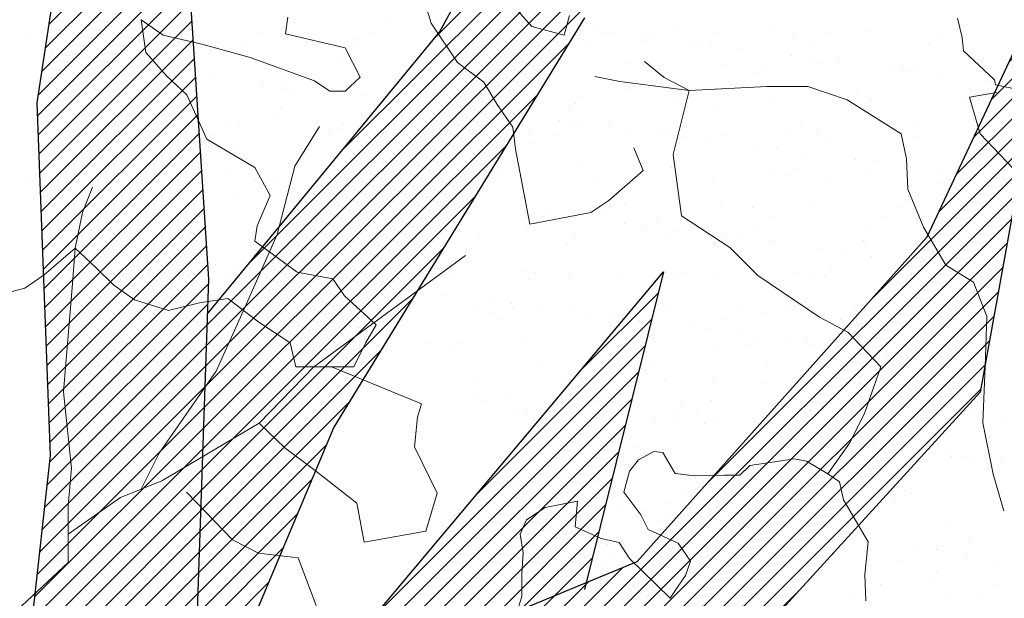
# Model space of a CAD drawing. Units: inches. Extents: x 1986 to 21484, y -1816 to 2016.
# Tile 33 of 85: x 2172.01 to 2182.74, y 1892.02 to 1898.33. Entities that reach past the tile are written whole.
import ezdxf

# ---------------------------------------------------------------- set-up
doc = ezdxf.new("R2010")
doc.units = ezdxf.units.IN
doc.layers.add('L-PLNT', color=84, linetype='Continuous', lineweight=13)
doc.layers.add('vfolhas', color=114, linetype='Continuous', lineweight=5)
doc.layers.add('vfolha2', color=110, linetype='Continuous')
doc.layers.add('vfolhas2', color=102, linetype='Continuous')
pattern_1 = [(45, (-2446.5133113, 50.986076), (-0.004419417382, 0.004419417382), [])]

# ---------------------------------------------------------------- blocks, each defined once
blk = doc.blocks.new('arbusto_PB_verde_grande')
at = {"layer": 'vfolha2'}
h = blk.add_hatch(dxfattribs=at)
h.set_pattern_fill('ANSI31', color=256, scale=0.05, style=0)
h.set_pattern_definition(pattern_1)
h.paths.add_polyline_path([(0.02944, 0.35651), (0.00028, 0.09048), (0.02625, -0.03934), (0.047, 0.06233), (0.06189, 0.09731), (0.09372, 0.26573), (0.09955, 0.43473), (0.08789, 0.61313), (0.0645, 0.72266), (0.04988, 0.6851), (0.0236, 0.51294)])
h.paths.add_polyline_path([(0.30106, 0.43789), (0.14225, 0.24871), (0.26685, 0.30022)])
h.paths.add_polyline_path([(0.37995, 0.22817), (0.23697, 0.15193), (0.18428, 0.09364), (0.11122, 0.04358), (0.02625, -0.03934), (0.28061, 0.04667), (0.36829, 0.07798), (0.46756, 0.11239), (0.61068, 0.19376), (0.71585, 0.27823), (0.55813, 0.25948)])
h.paths.add_polyline_path([(0.56101, -0.29441), (0.72752, -0.32573), (0.59024, -0.2412), (0.42962, -0.15982), (0.02625, -0.03934), (0.14922, -0.14107), (0.18838, -0.16604), (0.41501, -0.24435)])
h.paths.add_polyline_path([(-0.27429, -0.44776), (-0.30352, -0.72628), (-0.23923, -0.64175), (-0.15457, -0.45716), (0.02625, -0.03934), (-0.16328, -0.25376)])
h.paths.add_polyline_path([(-0.51963, -0.24744), (-0.67736, -0.32573), (-0.59558, -0.35072), (-0.40574, -0.32882), (-0.21007, -0.20995), (0.02625, -0.03934), (-0.14874, -0.06595), (-0.31518, -0.09101), (-0.41452, -0.15048)])
h.paths.add_polyline_path([(-0.52546, 0.25007), (-0.70947, 0.24698), (-0.51963, 0.1093), (-0.32979, 0.02167), (-0.07567, -0.0128), (-0.04234, -0.02148), (-0.35024, 0.1312)])
at = {"layer": 'vfolhas'}
h = blk.add_hatch(dxfattribs=at)
h.set_pattern_fill('ANSI31', color=256, scale=0.05, style=0)
h.set_pattern_definition(pattern_1)
h.paths.add_polyline_path([(-0.07279, 0.50669), (-0.18085, 0.65063), (-0.2334, 0.67253), (-0.20712, 0.53176), (-0.10785, 0.25007), (0.02625, -0.03934), (0.00028, 0.09048), (0.00816, 0.16241), (-0.04939, 0.29079)])
h.paths.add_polyline_path([(0.09902, 0.41929), (0.09372, 0.26573), (0.07906, 0.18814), (0.15506, 0.36901), (0.26606, 0.5505), (0.28356, 0.63504), (0.2485, 0.68819), (0.25145, 0.63504), (0.20178, 0.54426)])
h.paths.add_polyline_path([(0.12295, 0.24073), (0.047, 0.06233), (0.02625, -0.03934), (0.11122, 0.04358), (0.18428, 0.09364), (0.27478, 0.19376), (0.3215, 0.25323), (0.44129, 0.38467), (0.47634, 0.57866), (0.41789, 0.45347), (0.28939, 0.30954)])
h.paths.add_polyline_path([(0.58145, -0.03779), (0.70707, 0.01536), (0.78591, 0.04667), (0.74796, 0.06549), (0.62818, 0.08423), (0.52595, 0.09048), (0.39745, 0.04358), (0.02625, -0.03934), (0.25728, -0.03154), (0.43834, -0.0347)])
h.paths.add_polyline_path([(0.52022, -0.03647), (0.43834, -0.0347), (0.25728, -0.03154), (0.02625, -0.03934), (0.17964, -0.08515), (0.53768, -0.13167), (0.69541, -0.15357), (0.78591, -0.07852), (0.70413, -0.10042)])
h.paths.add_polyline_path([(0.27189, -0.21929), (0.14922, -0.14107), (0.02625, -0.03934), (0.15794, -0.31007), (0.29522, -0.42585), (0.41789, -0.49157), (0.56396, -0.56669), (0.5114, -0.48532), (0.39456, -0.34139)])
h.paths.add_polyline_path([(-0.05818, -0.47591), (-0.02312, -0.61984), (0.047, -0.80134), (0.08494, -0.59794), (0.07911, -0.4071), (0.03527, -0.25376), (0.02625, -0.03934), (-0.03773, -0.26001)])
h.paths.add_polyline_path([(-0.24218, 0.14054), (-0.11073, 0.06858), (0.02625, -0.03934), (-0.04235, 0.10871), (-0.21007, 0.23757), (-0.36485, 0.33145), (-0.47874, 0.40341), (-0.54303, 0.46288), (-0.49041, 0.33145), (-0.39408, 0.22192)])
at = {"layer": 'vfolha2'}
for p, q in [((0.0236, 0.51294), (0.04988, 0.6851)), ((0.08789, 0.61313), (0.09955, 0.43473)), ((0.02944, 0.35651), (0.0236, 0.51294)), ((0.14339, 0.25007), (0.30106, 0.43789)), ((0.30106, 0.43789), (0.26606, 0.29704)), ((0.09955, 0.43473), (0.09372, 0.26573)), ((0.00028, 0.09048), (0.02944, 0.35651))]:
    blk.add_line(p, q, dxfattribs=at)
at = {"layer": 'vfolhas2'}
for p, q in [((0.20178, 0.54426), (0.25145, 0.63504)), ((0.41789, 0.45347), (0.47634, 0.57866)), ((0.47634, 0.57866), (0.44129, 0.38467)), ((0.26606, 0.5505), (0.15506, 0.36901)), ((0.09902, 0.41929), (0.20178, 0.54426)), ((0.28939, 0.30954), (0.41789, 0.45347)), ((0.44129, 0.38467), (0.3215, 0.25323)), ((0.15506, 0.36901), (0.07795, 0.18551)), ((0.12295, 0.24073), (0.28939, 0.30954))]:
    blk.add_line(p, q, dxfattribs=at)
blk = doc.blocks.new('PLANT-SHRUB')
for p, q in [((2176.398, 1898.622), (2176.498, 1898.292)), ((2177.594, 1898.258), (2177.344, 1898.536)), ((2173.335, 1898.328), (2173.386, 1897.971)), ((2173.335, 1898.328), (2173.335, 1898.328)), ((2173.578, 1898.162), (2173.335, 1898.328)), ((2173.948, 1898.316), (2173.948, 1898.316)), ((2174.936, 1898.358), (2174.909, 1898.178)), ((2174.995, 1898.303), (2174.995, 1898.303)), ((2176.017, 1898.308), (2176.017, 1898.308)), ((2176.498, 1898.292), (2176.785, 1897.863)), ((2177.726, 1898.291), (2177.726, 1898.291)), ((2178.004, 1898.378), (2177.947, 1898.163)), ((2182.235, 1898.347), (2182.286, 1898.137)), ((2172.133, 1898.192), (2172.133, 1898.192)), ((2173.378, 1898.19), (2173.378, 1898.19)), ((2174.623, 1898.188), (2174.623, 1898.188)), ((2174.909, 1898.178), (2175.559, 1898.022)), ((2175.867, 1898.186), (2175.867, 1898.186)), ((2177.096, 1898.269), (2177.096, 1898.269)), ((2177.112, 1898.183), (2177.112, 1898.183)), ((2177.947, 1898.163), (2177.594, 1898.258)), ((2178.143, 1898.256), (2178.143, 1898.256)), ((2178.268, 1898.219), (2178.268, 1898.219)), ((2178.357, 1898.181), (2178.357, 1898.181)), ((2178.477, 1898.192), (2178.477, 1898.192)), ((2179.165, 1898.261), (2179.165, 1898.261)), ((2179.601, 1898.179), (2179.601, 1898.179)), ((2180.244, 1898.222), (2180.244, 1898.222)), ((2180.846, 1898.177), (2180.846, 1898.177)), ((2181.291, 1898.208), (2181.291, 1898.208)), ((2172.447, 1898.064), (2172.447, 1898.064)), ((2173.21, 1898.083), (2173.21, 1898.083)), ((2174.013, 1898.06), (2173.578, 1898.162)), ((2174.524, 1897.92), (2174.013, 1898.06)), ((2174.454, 1898.081), (2174.454, 1898.081)), ((2175.669, 1898.113), (2175.669, 1898.113)), ((2175.699, 1898.078), (2175.699, 1898.078)), ((2176.943, 1898.076), (2176.943, 1898.076)), ((2177.219, 1898.081), (2177.219, 1898.081)), ((2178.188, 1898.074), (2178.188, 1898.074)), ((2178.801, 1898.149), (2178.801, 1898.149)), ((2178.818, 1898.094), (2178.818, 1898.094)), ((2178.892, 1898.162), (2178.892, 1898.162)), ((2179.344, 1898.078), (2179.344, 1898.078)), ((2179.433, 1898.072), (2179.433, 1898.072)), ((2180.441, 1898.13), (2180.441, 1898.13)), ((2180.677, 1898.069), (2180.677, 1898.069)), ((2181.922, 1898.067), (2181.922, 1898.067)), ((2182.04, 1898.143), (2182.04, 1898.143)), ((2182.286, 1898.137), (2182.299, 1897.99)), ((2172.362, 1897.955), (2172.362, 1897.955)), ((2172.374, 1897.996), (2172.374, 1897.996)), ((2173.386, 1897.971), (2173.616, 1897.716)), ((2173.997, 1898.031), (2173.997, 1898.031)), ((2175.559, 1898.022), (2175.725, 1897.703)), ((2175.596, 1898.045), (2175.596, 1898.045)), ((2179.552, 1898.05), (2179.552, 1898.05)), ((2179.877, 1898.008), (2179.877, 1898.008)), ((2182.299, 1897.99), (2182.638, 1897.674)), ((2172.521, 1897.941), (2172.521, 1897.941)), ((2172.729, 1897.914), (2172.729, 1897.914)), ((2173.054, 1897.871), (2173.054, 1897.871)), ((2173.408, 1897.942), (2173.408, 1897.942)), ((2174.43, 1897.947), (2174.43, 1897.947)), ((2175.226, 1897.665), (2174.524, 1897.92)), ((2175.51, 1897.908), (2175.51, 1897.908)), ((2176.556, 1897.894), (2176.556, 1897.894)), ((2176.785, 1897.863), (2177.072, 1897.648)), ((2177.578, 1897.899), (2177.578, 1897.899)), ((2178.658, 1897.86), (2178.658, 1897.86)), ((2178.823, 1897.873), (2179.038, 1897.701)), ((2179.704, 1897.847), (2179.704, 1897.847)), ((2180.42, 1897.936), (2180.42, 1897.936)), ((2180.628, 1897.909), (2180.628, 1897.909)), ((2180.726, 1897.852), (2180.726, 1897.852)), ((2180.953, 1897.866), (2180.953, 1897.866)), ((2173.597, 1897.8), (2173.597, 1897.8)), ((2173.805, 1897.772), (2173.805, 1897.772)), ((2176.871, 1897.762), (2176.871, 1897.762)), ((2180.019, 1897.744), (2180.019, 1897.744)), ((2180.093, 1897.811), (2180.093, 1897.811)), ((2181.496, 1897.795), (2181.496, 1897.795)), ((2181.642, 1897.779), (2181.642, 1897.779)), ((2181.704, 1897.767), (2181.704, 1897.767)), ((2181.806, 1897.813), (2181.806, 1897.813)), ((2173.575, 1897.645), (2173.575, 1897.645)), ((2173.616, 1897.716), (2173.834, 1897.511)), ((2173.649, 1897.713), (2173.649, 1897.713)), ((2174.13, 1897.729), (2174.13, 1897.729)), ((2174.673, 1897.658), (2174.673, 1897.658)), ((2174.881, 1897.631), (2174.881, 1897.631)), ((2175.198, 1897.681), (2175.198, 1897.681)), ((2175.392, 1897.55), (2175.226, 1897.665)), ((2175.725, 1897.703), (2175.559, 1897.55)), ((2176.797, 1897.694), (2176.797, 1897.694)), ((2177.072, 1897.648), (2177.215, 1897.404)), ((2178.282, 1897.712), (2178.554, 1897.658)), ((2178.42, 1897.73), (2178.42, 1897.73)), ((2178.554, 1897.658), (2179.311, 1897.558)), ((2179.038, 1897.701), (2179.311, 1897.558)), ((2182.029, 1897.724), (2182.029, 1897.724)), ((2182.572, 1897.653), (2182.572, 1897.653)), ((2182.638, 1897.674), (2182.647, 1897.62)), ((2172.417, 1897.578), (2172.417, 1897.578)), ((2172.844, 1897.585), (2172.844, 1897.585)), ((2173.662, 1897.576), (2173.662, 1897.576)), ((2173.923, 1897.546), (2173.923, 1897.546)), ((2174.907, 1897.574), (2174.907, 1897.574)), ((2174.969, 1897.533), (2174.969, 1897.533)), ((2175.205, 1897.588), (2175.205, 1897.588)), ((2175.559, 1897.55), (2175.392, 1897.55)), ((2175.992, 1897.538), (2175.992, 1897.538)), ((2176.151, 1897.571), (2176.151, 1897.571)), ((2177.396, 1897.569), (2177.396, 1897.569)), ((2178.641, 1897.567), (2178.641, 1897.567)), ((2179.311, 1897.558), (2179.134, 1896.861)), ((2179.311, 1897.558), (2180.157, 1897.601)), ((2179.885, 1897.565), (2179.885, 1897.565)), ((2180.157, 1897.601), (2180.601, 1897.601)), ((2180.157, 1897.601), (2180.157, 1897.601)), ((2180.601, 1897.601), (2181.032, 1897.458)), ((2181.13, 1897.562), (2181.13, 1897.562)), ((2182.365, 1897.486), (2182.661, 1897.536)), ((2182.374, 1897.56), (2182.374, 1897.56)), ((2182.647, 1897.62), (2183.217, 1897.503)), ((2173.834, 1897.511), (2174.051, 1897.026)), ((2175.748, 1897.516), (2175.748, 1897.516)), ((2175.956, 1897.489), (2175.956, 1897.489)), ((2176.281, 1897.446), (2176.281, 1897.446)), ((2177.071, 1897.499), (2177.071, 1897.499)), ((2178.117, 1897.486), (2178.117, 1897.486)), ((2179.14, 1897.491), (2179.14, 1897.491)), ((2180.219, 1897.452), (2180.219, 1897.452)), ((2181.032, 1897.458), (2181.62, 1897.085)), ((2181.265, 1897.438), (2181.265, 1897.438)), ((2181.294, 1897.46), (2181.294, 1897.46)), ((2182.288, 1897.443), (2182.288, 1897.443)), ((2182.365, 1897.486), (2182.365, 1897.486)), ((2182.48, 1897.085), (2182.365, 1897.486)), ((2174.85, 1897.362), (2174.85, 1897.362)), ((2176.399, 1897.33), (2176.399, 1897.33)), ((2176.824, 1897.375), (2176.824, 1897.375)), ((2177.032, 1897.347), (2177.032, 1897.347)), ((2177.215, 1897.404), (2177.387, 1897.16)), ((2177.999, 1897.344), (2177.999, 1897.344)), ((2178.072, 1897.411), (2178.072, 1897.411)), ((2179.622, 1897.379), (2179.622, 1897.379)), ((2181.221, 1897.393), (2181.221, 1897.393)), ((2173.177, 1897.281), (2173.177, 1897.281)), ((2174.777, 1897.295), (2174.777, 1897.295)), ((2177.357, 1897.305), (2177.357, 1897.305)), ((2177.9, 1897.233), (2177.9, 1897.233)), ((2178.108, 1897.206), (2178.108, 1897.206)), ((2172.337, 1897.185), (2172.337, 1897.185)), ((2173.055, 1897.189), (2173.055, 1897.189)), ((2173.383, 1897.172), (2173.383, 1897.172)), ((2174.3, 1897.187), (2174.3, 1897.187)), ((2174.405, 1897.177), (2174.405, 1897.177)), ((2175.01, 1896.731), (2175.281, 1897.165)), ((2175.485, 1897.138), (2175.485, 1897.138)), ((2175.545, 1897.185), (2175.545, 1897.185)), ((2176.531, 1897.124), (2176.531, 1897.124)), ((2176.789, 1897.183), (2176.789, 1897.183)), ((2177.387, 1897.16), (2177.416, 1896.917)), ((2177.553, 1897.129), (2177.553, 1897.129)), ((2178.034, 1897.18), (2178.034, 1897.18)), ((2178.433, 1897.163), (2178.433, 1897.163)), ((2179.278, 1897.178), (2179.278, 1897.178)), ((2180.523, 1897.176), (2180.523, 1897.176)), ((2181.768, 1897.174), (2181.768, 1897.174)), ((2182.496, 1897.109), (2182.496, 1897.109)), ((2172.887, 1897.082), (2172.887, 1897.082)), ((2174.051, 1897.026), (2174.575, 1896.72)), ((2174.131, 1897.08), (2174.131, 1897.08)), ((2175.376, 1897.078), (2175.376, 1897.078)), ((2176.052, 1897.011), (2176.052, 1897.011)), ((2176.621, 1897.075), (2176.621, 1897.075)), ((2177.865, 1897.073), (2177.865, 1897.073)), ((2178.633, 1897.09), (2178.633, 1897.09)), ((2178.976, 1897.091), (2178.976, 1897.091)), ((2179.11, 1897.071), (2179.11, 1897.071)), ((2179.184, 1897.064), (2179.184, 1897.064)), ((2179.2, 1896.993), (2179.2, 1896.993)), ((2179.274, 1897.06), (2179.274, 1897.06)), ((2179.509, 1897.021), (2179.509, 1897.021)), ((2179.679, 1897.077), (2179.679, 1897.077)), ((2180.355, 1897.068), (2180.355, 1897.068)), ((2180.701, 1897.082), (2180.701, 1897.082)), ((2180.823, 1897.028), (2180.823, 1897.028)), ((2181.599, 1897.066), (2181.599, 1897.066)), ((2181.62, 1897.085), (2181.677, 1896.813)), ((2181.781, 1897.043), (2181.781, 1897.043)), ((2182.422, 1897.042), (2182.422, 1897.042)), ((2182.48, 1897.085), (2182.48, 1897.085)), ((2183.054, 1896.483), (2182.48, 1897.085)), ((2172.152, 1896.955), (2172.152, 1896.955)), ((2172.36, 1896.928), (2172.36, 1896.928)), ((2172.685, 1896.885), (2172.685, 1896.885)), ((2172.756, 1896.895), (2172.756, 1896.895)), ((2172.83, 1896.962), (2172.83, 1896.962)), ((2174.379, 1896.93), (2174.379, 1896.93)), ((2175.978, 1896.944), (2175.978, 1896.944)), ((2177.416, 1896.917), (2177.574, 1896.1)), ((2177.601, 1896.979), (2177.601, 1896.979)), ((2178.807, 1896.687), (2178.707, 1896.931)), ((2180.052, 1896.95), (2180.052, 1896.95)), ((2180.26, 1896.922), (2180.26, 1896.922)), ((2180.585, 1896.88), (2180.585, 1896.88)), ((2172.819, 1896.815), (2172.819, 1896.815)), ((2173.228, 1896.813), (2173.228, 1896.813)), ((2173.436, 1896.786), (2173.436, 1896.786)), ((2173.898, 1896.776), (2173.898, 1896.776)), ((2179.134, 1896.861), (2179.225, 1896.191)), ((2181.127, 1896.808), (2181.127, 1896.808)), ((2181.335, 1896.781), (2181.335, 1896.781)), ((2181.677, 1896.813), (2181.691, 1896.483)), ((2173.761, 1896.743), (2173.761, 1896.743)), ((2174.304, 1896.672), (2174.304, 1896.672)), ((2174.575, 1896.72), (2174.741, 1896.413)), ((2174.82, 1895.986), (2175.01, 1896.731)), ((2174.944, 1896.763), (2174.944, 1896.763)), ((2175.967, 1896.768), (2175.967, 1896.768)), ((2177.046, 1896.729), (2177.046, 1896.729)), ((2178.092, 1896.716), (2178.092, 1896.716)), ((2178.434, 1896.358), (2178.807, 1896.687)), ((2178.807, 1896.687), (2178.807, 1896.687)), ((2179.115, 1896.72), (2179.115, 1896.72)), ((2180.194, 1896.682), (2180.194, 1896.682)), ((2180.475, 1896.71), (2180.475, 1896.71)), ((2181.24, 1896.668), (2181.24, 1896.668)), ((2181.66, 1896.738), (2181.66, 1896.738)), ((2182.024, 1896.677), (2182.024, 1896.677)), ((2182.203, 1896.667), (2182.203, 1896.667)), ((2182.263, 1896.673), (2182.263, 1896.673)), ((2172.095, 1896.577), (2172.095, 1896.577)), ((2173.339, 1896.575), (2173.339, 1896.575)), ((2174.031, 1896.611), (2174.031, 1896.611)), ((2174.512, 1896.644), (2174.512, 1896.644)), ((2174.584, 1896.573), (2174.584, 1896.573)), ((2174.837, 1896.602), (2174.837, 1896.602)), ((2175.58, 1896.579), (2175.58, 1896.579)), ((2175.828, 1896.571), (2175.828, 1896.571)), ((2177.073, 1896.568), (2177.073, 1896.568)), ((2177.18, 1896.593), (2177.18, 1896.593)), ((2177.253, 1896.661), (2177.253, 1896.661)), ((2178.318, 1896.566), (2178.318, 1896.566)), ((2178.802, 1896.628), (2178.802, 1896.628)), ((2179.562, 1896.564), (2179.562, 1896.564)), ((2180.402, 1896.642), (2180.402, 1896.642)), ((2180.807, 1896.562), (2180.807, 1896.562)), ((2182.052, 1896.559), (2182.052, 1896.559)), ((2182.411, 1896.639), (2182.411, 1896.639)), ((2182.736, 1896.596), (2182.736, 1896.596)), ((2172.358, 1896.53), (2172.358, 1896.53)), ((2172.697, 1896.226), (2172.806, 1896.504)), ((2173.957, 1896.544), (2173.957, 1896.544)), ((2175.38, 1896.53), (2175.38, 1896.53)), ((2175.588, 1896.503), (2175.588, 1896.503)), ((2175.913, 1896.46), (2175.913, 1896.46)), ((2181.691, 1896.483), (2181.863, 1896.067)), ((2172.311, 1896.415), (2172.311, 1896.415)), ((2173.358, 1896.402), (2173.358, 1896.402)), ((2174.38, 1896.406), (2174.38, 1896.406)), ((2174.741, 1896.413), (2174.6, 1896.081)), ((2175.459, 1896.368), (2175.459, 1896.368)), ((2176.456, 1896.388), (2176.456, 1896.388)), ((2176.506, 1896.354), (2176.506, 1896.354)), ((2176.664, 1896.361), (2176.664, 1896.361)), ((2177.528, 1896.359), (2177.528, 1896.359)), ((2178.239, 1896.228), (2178.434, 1896.358)), ((2181.677, 1896.359), (2181.677, 1896.359)), ((2175.233, 1896.261), (2175.233, 1896.261)), ((2176.989, 1896.318), (2176.989, 1896.318)), ((2177.531, 1896.247), (2177.531, 1896.247)), ((2178.381, 1896.242), (2178.381, 1896.242)), ((2178.455, 1896.31), (2178.455, 1896.31)), ((2178.608, 1896.32), (2178.608, 1896.32)), ((2179.654, 1896.307), (2179.654, 1896.307)), ((2180.004, 1896.278), (2180.004, 1896.278)), ((2180.676, 1896.312), (2180.676, 1896.312)), ((2181.603, 1896.291), (2181.603, 1896.291)), ((2181.756, 1896.273), (2181.756, 1896.273)), ((2172.618, 1895.838), (2172.697, 1896.226)), ((2172.732, 1896.189), (2172.732, 1896.189)), ((2173.56, 1896.179), (2173.56, 1896.179)), ((2173.977, 1896.186), (2173.977, 1896.186)), ((2175.159, 1896.193), (2175.159, 1896.193)), ((2175.222, 1896.184), (2175.222, 1896.184)), ((2176.466, 1896.182), (2176.466, 1896.182)), ((2176.782, 1896.228), (2176.782, 1896.228)), ((2177.574, 1896.1), (2178.239, 1896.228)), ((2177.711, 1896.18), (2177.711, 1896.18)), ((2177.74, 1896.219), (2177.74, 1896.219)), ((2178.064, 1896.177), (2178.064, 1896.177)), ((2178.956, 1896.177), (2178.956, 1896.177)), ((2179.225, 1896.191), (2179.751, 1895.847)), ((2180.2, 1896.175), (2180.2, 1896.175)), ((2181.445, 1896.173), (2181.445, 1896.173)), ((2182.69, 1896.17), (2182.69, 1896.17)), ((2172.564, 1896.081), (2172.564, 1896.081)), ((2172.793, 1896.045), (2172.793, 1896.045)), ((2173.809, 1896.079), (2173.809, 1896.079)), ((2174.6, 1896.081), (2174.575, 1895.915)), ((2175.053, 1896.077), (2175.053, 1896.077)), ((2176.298, 1896.074), (2176.298, 1896.074)), ((2177.542, 1896.072), (2177.542, 1896.072)), ((2178.607, 1896.105), (2178.607, 1896.105)), ((2178.787, 1896.07), (2178.787, 1896.07)), ((2178.815, 1896.078), (2178.815, 1896.078)), ((2179.14, 1896.035), (2179.14, 1896.035)), ((2180.032, 1896.068), (2180.032, 1896.068)), ((2181.276, 1896.065), (2181.276, 1896.065)), ((2181.863, 1896.067), (2182.107, 1895.652)), ((2182.521, 1896.063), (2182.521, 1896.063)), ((2173.873, 1896.006), (2173.873, 1896.006)), ((2174.451, 1895.16), (2174.82, 1895.986)), ((2174.575, 1895.915), (2175.036, 1895.577)), ((2174.919, 1895.993), (2174.919, 1895.993)), ((2175.941, 1895.998), (2175.941, 1895.998)), ((2177.021, 1895.959), (2177.021, 1895.959)), ((2178.067, 1895.945), (2178.067, 1895.945)), ((2179.089, 1895.95), (2179.089, 1895.95)), ((2179.656, 1895.959), (2179.656, 1895.959)), ((2179.683, 1895.964), (2179.683, 1895.964)), ((2179.891, 1895.936), (2179.891, 1895.936)), ((2181.205, 1895.927), (2181.205, 1895.927)), ((2172.618, 1895.838), (2172.279, 1895.547)), ((2172.317, 1895.899), (2172.317, 1895.899)), ((2172.588, 1895.453), (2172.618, 1895.838)), ((2172.618, 1895.838), (2172.618, 1895.838)), ((2172.844, 1895.628), (2172.618, 1895.838)), ((2172.86, 1895.827), (2172.86, 1895.827)), ((2173.212, 1895.861), (2173.212, 1895.861)), ((2174.761, 1895.829), (2174.761, 1895.829)), ((2176.36, 1895.842), (2176.36, 1895.842)), ((2176.434, 1895.91), (2176.434, 1895.91)), ((2177.983, 1895.878), (2177.983, 1895.878)), ((2179.582, 1895.891), (2179.582, 1895.891)), ((2179.751, 1895.847), (2180.059, 1895.539)), ((2180.169, 1895.912), (2180.169, 1895.912)), ((2180.216, 1895.893), (2180.216, 1895.893)), ((2180.759, 1895.822), (2180.759, 1895.822)), ((2181.215, 1895.898), (2181.215, 1895.898)), ((2182.238, 1895.903), (2182.238, 1895.903)), ((2173.068, 1895.8), (2173.068, 1895.8)), ((2173.138, 1895.793), (2173.138, 1895.793)), ((2173.393, 1895.757), (2173.393, 1895.757)), ((2175.217, 1894.543), (2176.872, 1895.76)), ((2180.967, 1895.795), (2180.967, 1895.795)), ((2181.292, 1895.752), (2181.292, 1895.752)), ((2172.286, 1895.645), (2172.286, 1895.645)), ((2173.038, 1895.434), (2172.844, 1895.628)), ((2173.269, 1895.643), (2173.269, 1895.643)), ((2173.936, 1895.685), (2173.936, 1895.685)), ((2174.144, 1895.658), (2174.144, 1895.658)), ((2174.355, 1895.636), (2174.355, 1895.636)), ((2174.468, 1895.615), (2174.468, 1895.615)), ((2175.434, 1895.597), (2175.434, 1895.597)), ((2180.858, 1895.608), (2180.858, 1895.608)), ((2181.835, 1895.68), (2181.835, 1895.68)), ((2182.043, 1895.653), (2182.043, 1895.653)), ((2182.107, 1895.652), (2182.408, 1895.466)), ((2182.368, 1895.61), (2182.368, 1895.61)), ((2172.279, 1895.547), (2172.069, 1895.402)), ((2172.982, 1895.523), (2172.982, 1895.523)), ((2173.017, 1895.558), (2173.017, 1895.558)), ((2173.11, 1895.497), (2173.11, 1895.497)), ((2173.426, 1895.56), (2173.426, 1895.56)), ((2173.479, 1895.522), (2173.479, 1895.522)), ((2173.75, 1895.503), (2173.75, 1895.503)), ((2173.779, 1895.53), (2173.779, 1895.53)), ((2173.858, 1895.544), (2173.858, 1895.544)), ((2173.977, 1895.521), (2173.977, 1895.521)), ((2174.276, 1895.539), (2174.276, 1895.539)), ((2174.399, 1895.517), (2174.399, 1895.517)), ((2174.475, 1895.521), (2174.475, 1895.521)), ((2175.011, 1895.544), (2175.011, 1895.544)), ((2175.036, 1895.577), (2175.424, 1895.505)), ((2175.219, 1895.516), (2175.219, 1895.516)), ((2175.424, 1895.505), (2175.553, 1895.318)), ((2175.506, 1895.57), (2175.506, 1895.57)), ((2176.48, 1895.584), (2176.48, 1895.584)), ((2176.75, 1895.568), (2176.75, 1895.568)), ((2177.503, 1895.589), (2177.503, 1895.589)), ((2177.562, 1895.492), (2177.562, 1895.492)), ((2177.635, 1895.559), (2177.635, 1895.559)), ((2177.995, 1895.565), (2177.995, 1895.565)), ((2178.582, 1895.55), (2178.582, 1895.55)), ((2179.185, 1895.527), (2179.185, 1895.527)), ((2179.24, 1895.563), (2179.24, 1895.563)), ((2179.629, 1895.537), (2179.629, 1895.537)), ((2180.059, 1895.539), (2180.729, 1895.086)), ((2180.484, 1895.561), (2180.484, 1895.561)), ((2180.651, 1895.542), (2180.651, 1895.542)), ((2180.784, 1895.541), (2180.784, 1895.541)), ((2181.729, 1895.558), (2181.729, 1895.558)), ((2181.73, 1895.503), (2181.73, 1895.503)), ((2182.407, 1895.576), (2182.407, 1895.576)), ((2172.069, 1895.402), (2171.585, 1895.273)), ((2172.491, 1894.27), (2172.588, 1895.453)), ((2173.264, 1895.273), (2173.038, 1895.434)), ((2173.135, 1895.377), (2173.135, 1895.377)), ((2173.223, 1895.4), (2173.223, 1895.4)), ((2173.412, 1895.479), (2173.412, 1895.479)), ((2173.642, 1895.394), (2173.642, 1895.394)), ((2173.91, 1895.478), (2173.91, 1895.478)), ((2174.051, 1895.396), (2174.051, 1895.396)), ((2174.26, 1895.39), (2174.26, 1895.39)), ((2174.408, 1895.478), (2174.408, 1895.478)), ((2174.482, 1895.381), (2174.482, 1895.381)), ((2175.544, 1895.474), (2175.544, 1895.474)), ((2175.963, 1895.478), (2175.963, 1895.478)), ((2176.087, 1895.402), (2176.087, 1895.402)), ((2182.408, 1895.466), (2182.552, 1895.093)), ((2173.635, 1895.16), (2173.264, 1895.273)), ((2173.265, 1895.36), (2173.265, 1895.36)), ((2173.483, 1895.331), (2173.483, 1895.331)), ((2173.566, 1895.32), (2173.566, 1895.32)), ((2173.591, 1895.357), (2173.591, 1895.357)), ((2173.593, 1895.277), (2173.593, 1895.277)), ((2173.696, 1895.303), (2173.696, 1895.303)), ((2173.913, 1895.274), (2173.913, 1895.274)), ((2174.281, 1895.289), (2173.974, 1895.241)), ((2174.091, 1895.276), (2174.091, 1895.276)), ((2174.231, 1895.363), (2174.231, 1895.363)), ((2174.281, 1895.289), (2174.281, 1895.289)), ((2174.62, 1895.031), (2174.281, 1895.289)), ((2174.589, 1895.275), (2174.589, 1895.275)), ((2175.553, 1895.318), (2175.898, 1895.003)), ((2176.295, 1895.375), (2176.295, 1895.375)), ((2176.62, 1895.332), (2176.62, 1895.332)), ((2173.416, 1895.252), (2173.416, 1895.252)), ((2173.452, 1895.23), (2173.452, 1895.23)), ((2173.974, 1895.241), (2173.635, 1895.16)), ((2173.848, 1895.236), (2173.848, 1895.236)), ((2173.974, 1895.241), (2173.974, 1895.241)), ((2173.996, 1895.264), (2173.996, 1895.264)), ((2174.426, 1895.207), (2174.426, 1895.207)), ((2174.556, 1895.19), (2174.556, 1895.19)), ((2174.894, 1895.223), (2174.894, 1895.223)), ((2174.899, 1895.183), (2174.899, 1895.183)), ((2175.916, 1895.228), (2175.916, 1895.228)), ((2176.144, 1895.181), (2176.144, 1895.181)), ((2176.996, 1895.189), (2176.996, 1895.189)), ((2177.163, 1895.261), (2177.163, 1895.261)), ((2177.371, 1895.233), (2177.371, 1895.233)), ((2177.388, 1895.179), (2177.388, 1895.179)), ((2177.696, 1895.19), (2177.696, 1895.19)), ((2178.042, 1895.175), (2178.042, 1895.175)), ((2178.633, 1895.176), (2178.633, 1895.176)), ((2178.837, 1895.208), (2178.837, 1895.208)), ((2179.064, 1895.18), (2179.064, 1895.18)), ((2179.878, 1895.174), (2179.878, 1895.174)), ((2180.386, 1895.176), (2180.386, 1895.176)), ((2181.122, 1895.172), (2181.122, 1895.172)), ((2181.985, 1895.19), (2181.985, 1895.19)), ((2182.059, 1895.257), (2182.059, 1895.257)), ((2182.367, 1895.17), (2182.367, 1895.17)), ((2174.155, 1894.495), (2174.451, 1895.16)), ((2174.73, 1895.076), (2174.73, 1895.076)), ((2175.541, 1895.092), (2175.541, 1895.092)), ((2175.615, 1895.159), (2175.615, 1895.159)), ((2175.975, 1895.074), (2175.975, 1895.074)), ((2177.164, 1895.127), (2177.164, 1895.127)), ((2177.22, 1895.071), (2177.22, 1895.071)), ((2178.239, 1895.119), (2178.239, 1895.119)), ((2178.447, 1895.092), (2178.447, 1895.092)), ((2178.464, 1895.069), (2178.464, 1895.069)), ((2178.763, 1895.141), (2178.763, 1895.141)), ((2179.709, 1895.067), (2179.709, 1895.067)), ((2180.144, 1895.141), (2180.144, 1895.141)), ((2180.729, 1895.086), (2181.037, 1894.923)), ((2180.954, 1895.065), (2180.954, 1895.065)), ((2181.19, 1895.128), (2181.19, 1895.128)), ((2182.198, 1895.062), (2182.198, 1895.062)), ((2182.212, 1895.133), (2182.212, 1895.133)), ((2182.552, 1895.093), (2182.537, 1894.548)), ((2174.959, 1894.805), (2174.62, 1895.031)), ((2175.702, 1894.969), (2175.702, 1894.969)), ((2175.898, 1895.003), (2175.783, 1894.802)), ((2175.847, 1895.02), (2175.847, 1895.02)), ((2178.772, 1895.049), (2178.772, 1895.049)), ((2179.315, 1894.977), (2179.315, 1894.977)), ((2179.523, 1894.95), (2179.523, 1894.95)), ((2174.957, 1894.874), (2174.957, 1894.874)), ((2175.033, 1894.936), (2175.033, 1894.936)), ((2175.097, 1894.909), (2175.097, 1894.909)), ((2175.455, 1894.873), (2175.455, 1894.873)), ((2175.515, 1894.904), (2175.515, 1894.904)), ((2175.672, 1894.942), (2175.672, 1894.942)), ((2179.848, 1894.907), (2179.848, 1894.907)), ((2180.038, 1894.858), (2180.038, 1894.858)), ((2181.037, 1894.923), (2181.4, 1894.543)), ((2175.024, 1894.543), (2174.959, 1894.805)), ((2175.29, 1894.761), (2175.29, 1894.761)), ((2175.513, 1894.796), (2175.513, 1894.796)), ((2175.783, 1894.802), (2175.654, 1894.543)), ((2175.721, 1894.746), (2175.721, 1894.746)), ((2176.455, 1894.814), (2176.455, 1894.814)), ((2176.743, 1894.741), (2176.743, 1894.741)), ((2176.816, 1894.808), (2176.816, 1894.808)), ((2177.478, 1894.819), (2177.478, 1894.819)), ((2178.365, 1894.776), (2178.365, 1894.776)), ((2178.557, 1894.78), (2178.557, 1894.78)), ((2179.603, 1894.767), (2179.603, 1894.767)), ((2179.965, 1894.79), (2179.965, 1894.79)), ((2180.39, 1894.836), (2180.39, 1894.836)), ((2180.598, 1894.808), (2180.598, 1894.808)), ((2180.626, 1894.772), (2180.626, 1894.772)), ((2180.923, 1894.765), (2180.923, 1894.765)), ((2181.588, 1894.825), (2181.588, 1894.825)), ((2181.705, 1894.733), (2181.705, 1894.733)), ((2175.057, 1894.71), (2175.057, 1894.71)), ((2175.14, 1894.699), (2175.14, 1894.699)), ((2175.145, 1894.675), (2175.145, 1894.675)), ((2175.213, 1894.718), (2175.213, 1894.718)), ((2175.27, 1894.682), (2175.27, 1894.682)), ((2175.345, 1894.641), (2175.345, 1894.641)), ((2175.374, 1894.668), (2175.374, 1894.668)), ((2175.487, 1894.653), (2175.487, 1894.653)), ((2175.57, 1894.642), (2175.57, 1894.642)), ((2175.643, 1894.674), (2175.643, 1894.674)), ((2175.71, 1894.717), (2175.71, 1894.717)), ((2181.466, 1894.694), (2181.466, 1894.694)), ((2181.674, 1894.667), (2181.674, 1894.667)), ((2174.624, 1893.928), (2175.217, 1894.543)), ((2175.41, 1894.543), (2175.024, 1894.543)), ((2175.087, 1894.601), (2175.087, 1894.601)), ((2175.41, 1894.543), (2176.393, 1894.141)), ((2175.654, 1894.543), (2175.41, 1894.543)), ((2175.505, 1894.596), (2175.505, 1894.596)), ((2177.672, 1894.564), (2177.672, 1894.564)), ((2178.917, 1894.562), (2178.917, 1894.562)), ((2180.161, 1894.56), (2180.161, 1894.56)), ((2181.4, 1894.543), (2181.219, 1894.036)), ((2181.406, 1894.558), (2181.406, 1894.558)), ((2181.999, 1894.624), (2181.999, 1894.624)), ((2182.537, 1894.548), (2182.509, 1893.932)), ((2182.542, 1894.552), (2182.542, 1894.552)), ((2182.651, 1894.555), (2182.651, 1894.555)), ((2173.532, 1893.601), (2174.155, 1894.495)), ((2176.971, 1894.419), (2176.971, 1894.419)), ((2178.018, 1894.458), (2178.018, 1894.458)), ((2179.039, 1894.41), (2179.039, 1894.41)), ((2179.567, 1894.426), (2179.567, 1894.426)), ((2181.166, 1894.439), (2181.166, 1894.439)), ((2181.24, 1894.507), (2181.24, 1894.507)), ((2177.944, 1894.39), (2177.944, 1894.39)), ((2178.017, 1894.405), (2178.017, 1894.405)), ((2180.119, 1894.371), (2180.119, 1894.371)), ((2181.165, 1894.358), (2181.165, 1894.358)), ((2182.187, 1894.363), (2182.187, 1894.363)), ((2172.576, 1893.437), (2172.491, 1894.27)), ((2177.003, 1894.247), (2177.003, 1894.247)), ((2177.327, 1894.204), (2177.327, 1894.204)), ((2176.393, 1894.141), (2176.348, 1893.995)), ((2177.065, 1894.178), (2177.065, 1894.178)), ((2177.87, 1894.133), (2177.87, 1894.133)), ((2178.078, 1894.105), (2178.078, 1894.105)), ((2178.31, 1894.176), (2178.31, 1894.176)), ((2179.219, 1894.107), (2179.219, 1894.107)), ((2179.555, 1894.173), (2179.555, 1894.173)), ((2180.799, 1894.171), (2180.799, 1894.171)), ((2182.044, 1894.169), (2182.044, 1894.169)), ((2182.368, 1894.088), (2182.368, 1894.088)), ((2182.441, 1894.156), (2182.441, 1894.156)), ((2176.348, 1893.995), (2176.315, 1893.671)), ((2177.453, 1894.049), (2177.453, 1894.049)), ((2177.546, 1894.026), (2177.546, 1894.026)), ((2178.142, 1894.068), (2178.142, 1894.068)), ((2178.403, 1894.062), (2178.403, 1894.062)), ((2178.532, 1894.01), (2178.532, 1894.01)), ((2178.946, 1893.991), (2178.946, 1893.991)), ((2179.146, 1894.039), (2179.146, 1894.039)), ((2179.386, 1894.066), (2179.386, 1894.066)), ((2179.578, 1893.997), (2179.578, 1893.997)), ((2180.601, 1894.001), (2180.601, 1894.001)), ((2180.631, 1894.064), (2180.631, 1894.064)), ((2180.768, 1894.075), (2180.768, 1894.075)), ((2181.219, 1894.036), (2181.056, 1893.71)), ((2181.875, 1894.061), (2181.875, 1894.061)), ((2173.563, 1893.3), (2174.624, 1893.928)), ((2174.904, 1893.66), (2174.624, 1893.928)), ((2179.154, 1893.964), (2179.154, 1893.964)), ((2179.479, 1893.921), (2179.479, 1893.921)), ((2181.68, 1893.963), (2181.68, 1893.963)), ((2182.509, 1893.932), (2182.624, 1893.373)), ((2182.726, 1893.949), (2182.726, 1893.949)), ((2180.022, 1893.849), (2180.022, 1893.849)), ((2180.23, 1893.822), (2180.23, 1893.822)), ((2180.555, 1893.779), (2180.555, 1893.779)), ((2175.217, 1893.425), (2174.904, 1893.66)), ((2176.315, 1893.671), (2176.561, 1893.167)), ((2178.748, 1893.675), (2178.748, 1893.675)), ((2180.347, 1893.689), (2180.347, 1893.689)), ((2180.421, 1893.756), (2180.421, 1893.756)), ((2181.056, 1893.71), (2180.822, 1893.378)), ((2181.098, 1893.708), (2181.098, 1893.708)), ((2181.306, 1893.68), (2181.306, 1893.68)), ((2181.97, 1893.724), (2181.97, 1893.724)), ((2173.338, 1893.209), (2173.532, 1893.601)), ((2177.349, 1893.564), (2177.349, 1893.564)), ((2177.992, 1893.635), (2177.992, 1893.635)), ((2178.594, 1893.561), (2178.594, 1893.561)), ((2178.925, 1893.619), (2178.757, 1893.53)), ((2179.023, 1893.61), (2178.925, 1893.619)), ((2179.014, 1893.64), (2179.014, 1893.64)), ((2179.155, 1893.38), (2179.023, 1893.61)), ((2179.839, 1893.559), (2179.839, 1893.559)), ((2180.093, 1893.601), (2180.093, 1893.601)), ((2181.083, 1893.557), (2181.083, 1893.557)), ((2181.14, 1893.588), (2181.14, 1893.588)), ((2181.631, 1893.638), (2181.631, 1893.638)), ((2182.162, 1893.593), (2182.162, 1893.593)), ((2182.174, 1893.566), (2182.174, 1893.566)), ((2182.328, 1893.555), (2182.328, 1893.555)), ((2178.757, 1893.53), (2178.66, 1893.407)), ((2179.969, 1893.468), (2179.863, 1893.362)), ((2180.456, 1893.539), (2179.969, 1893.468)), ((2180.588, 1893.513), (2180.456, 1893.539)), ((2180.822, 1893.378), (2180.588, 1893.513)), ((2182.382, 1893.539), (2182.382, 1893.539)), ((2182.707, 1893.496), (2182.707, 1893.496)), ((2172.54, 1893.026), (2172.576, 1893.437)), ((2175.688, 1893.055), (2175.217, 1893.425)), ((2178.4, 1893.356), (2178.4, 1893.356)), ((2178.66, 1893.407), (2178.598, 1893.177)), ((2179.368, 1893.353), (2179.155, 1893.38)), ((2179.695, 1893.362), (2179.368, 1893.353)), ((2179.695, 1893.362), (2179.695, 1893.362)), ((2179.863, 1893.362), (2179.695, 1893.362)), ((2179.863, 1893.362), (2179.863, 1893.362)), ((2180.822, 1893.378), (2180.822, 1893.378)), ((2180.822, 1893.378), (2180.948, 1893.289)), ((2181.548, 1893.338), (2181.548, 1893.338)), ((2181.622, 1893.405), (2181.622, 1893.405)), ((2182.624, 1893.373), (2182.738, 1892.972)), ((2173.113, 1893.118), (2173.563, 1893.3)), ((2177.427, 1893.279), (2177.427, 1893.279)), ((2178.326, 1893.289), (2178.326, 1893.289)), ((2178.507, 1893.24), (2178.507, 1893.24)), ((2179.949, 1893.324), (2179.949, 1893.324)), ((2180.575, 1893.231), (2180.575, 1893.231)), ((2180.948, 1893.289), (2180.993, 1893.092)), ((2173.83, 1893.175), (2174.331, 1892.656)), ((2176.561, 1893.167), (2176.438, 1892.753)), ((2177.502, 1893.146), (2177.502, 1893.146)), ((2177.987, 1893.175), (2177.987, 1893.175)), ((2178.598, 1893.177), (2178.784, 1892.929)), ((2179.232, 1893.173), (2179.232, 1893.173)), ((2179.553, 1893.226), (2179.553, 1893.226)), ((2180.477, 1893.17), (2180.477, 1893.17)), ((2181.655, 1893.193), (2181.655, 1893.193)), ((2181.721, 1893.168), (2181.721, 1893.168)), ((2182.701, 1893.179), (2182.701, 1893.179)), ((2172.54, 1892.718), (2173.113, 1893.118)), ((2172.54, 1892.411), (2172.54, 1893.026)), ((2175.766, 1892.63), (2175.688, 1893.055)), ((2177.71, 1893.119), (2177.71, 1893.119)), ((2178.094, 1893.079), (2177.74, 1893.009)), ((2177.819, 1893.067), (2177.819, 1893.067)), ((2177.973, 1893.018), (2177.973, 1893.018)), ((2178.035, 1893.076), (2178.035, 1893.076)), ((2178.053, 1893.059), (2178.053, 1893.059)), ((2178.067, 1892.797), (2178.094, 1893.079)), ((2178.094, 1893.079), (2178.094, 1893.079)), ((2179.063, 1893.065), (2179.063, 1893.065)), ((2180.308, 1893.063), (2180.308, 1893.063)), ((2180.993, 1893.092), (2181.261, 1892.636)), ((2181.553, 1893.061), (2181.553, 1893.061)), ((2177.74, 1893.009), (2177.537, 1892.876)), ((2177.894, 1892.913), (2177.894, 1892.913)), ((2177.929, 1892.924), (2177.929, 1892.924)), ((2178.578, 1893.005), (2178.578, 1893.005)), ((2178.784, 1892.929), (2178.864, 1892.77)), ((2178.786, 1892.977), (2178.786, 1892.977)), ((2179.111, 1892.935), (2179.111, 1892.935)), ((2179.528, 1892.938), (2179.528, 1892.938)), ((2179.602, 1893.005), (2179.602, 1893.005)), ((2181.151, 1892.973), (2181.151, 1892.973)), ((2177.537, 1892.876), (2177.466, 1892.717)), ((2177.748, 1892.875), (2177.748, 1892.875)), ((2177.797, 1892.866), (2177.797, 1892.866)), ((2177.966, 1892.865), (2177.966, 1892.865)), ((2178.989, 1892.87), (2178.989, 1892.87)), ((2179.653, 1892.863), (2179.653, 1892.863)), ((2179.862, 1892.836), (2179.862, 1892.836)), ((2180.068, 1892.831), (2180.068, 1892.831)), ((2181.114, 1892.818), (2181.114, 1892.818)), ((2182.137, 1892.823), (2182.137, 1892.823)), ((2176.438, 1892.753), (2175.766, 1892.63)), ((2177.466, 1892.717), (2177.501, 1892.514)), ((2177.479, 1892.735), (2177.479, 1892.735)), ((2177.545, 1892.715), (2177.545, 1892.715)), ((2177.554, 1892.711), (2177.554, 1892.711)), ((2177.562, 1892.724), (2177.562, 1892.724)), ((2177.692, 1892.707), (2177.692, 1892.707)), ((2177.726, 1892.758), (2177.726, 1892.758)), ((2177.755, 1892.785), (2177.755, 1892.785)), ((2177.963, 1892.71), (2177.963, 1892.71)), ((2178.052, 1892.71), (2178.052, 1892.71)), ((2178.35, 1892.673), (2178.067, 1892.797)), ((2178.864, 1892.77), (2179.191, 1892.62)), ((2180.186, 1892.793), (2180.186, 1892.793)), ((2180.729, 1892.721), (2180.729, 1892.721)), ((2180.937, 1892.694), (2180.937, 1892.694)), ((2174.331, 1892.656), (2174.617, 1892.513)), ((2177.487, 1892.668), (2177.487, 1892.668)), ((2177.567, 1892.613), (2177.567, 1892.613)), ((2177.581, 1892.606), (2177.581, 1892.606)), ((2177.91, 1892.679), (2177.91, 1892.679)), ((2177.985, 1892.667), (2177.985, 1892.667)), ((2177.993, 1892.668), (2177.993, 1892.668)), ((2178.123, 1892.651), (2178.123, 1892.651)), ((2178.206, 1892.618), (2178.206, 1892.618)), ((2178.236, 1892.645), (2178.236, 1892.645)), ((2178.34, 1892.622), (2178.34, 1892.622)), ((2178.545, 1892.629), (2178.35, 1892.673)), ((2178.423, 1892.611), (2178.423, 1892.611)), ((2178.66, 1892.452), (2178.545, 1892.629)), ((2178.553, 1892.594), (2178.553, 1892.594)), ((2179.191, 1892.62), (2179.323, 1892.425)), ((2180.729, 1892.587), (2180.729, 1892.587)), ((2180.803, 1892.655), (2180.803, 1892.655)), ((2181.261, 1892.636), (2181.225, 1892.278)), ((2181.262, 1892.651), (2181.262, 1892.651)), ((2182.352, 1892.623), (2182.352, 1892.623)), ((2174.617, 1892.513), (2175.047, 1892.46)), ((2177.027, 1892.563), (2177.027, 1892.563)), ((2177.402, 1892.509), (2177.402, 1892.509)), ((2177.501, 1892.514), (2177.484, 1892.284)), ((2177.507, 1892.538), (2177.507, 1892.538)), ((2177.738, 1892.567), (2177.738, 1892.567)), ((2178.169, 1892.551), (2178.169, 1892.551)), ((2178.271, 1892.561), (2178.271, 1892.561)), ((2178.588, 1892.546), (2178.588, 1892.546)), ((2179.13, 1892.573), (2179.13, 1892.573)), ((2179.516, 1892.558), (2179.516, 1892.558)), ((2180.761, 1892.556), (2180.761, 1892.556)), ((2181.805, 1892.58), (2181.805, 1892.58)), ((2182.005, 1892.554), (2182.005, 1892.554)), ((2182.013, 1892.552), (2182.013, 1892.552)), ((2182.338, 1892.51), (2182.338, 1892.51)), ((2171.837, 1891.752), (2172.54, 1892.411)), ((2175.047, 1892.46), (2175.244, 1891.941)), ((2177.535, 1892.407), (2177.535, 1892.407)), ((2177.668, 1892.465), (2177.668, 1892.465)), ((2177.953, 1892.402), (2177.953, 1892.402)), ((2178.047, 1892.472), (2178.047, 1892.472)), ((2178.166, 1892.464), (2178.166, 1892.464)), ((2178.362, 1892.404), (2178.362, 1892.404)), ((2178.482, 1892.47), (2178.482, 1892.47)), ((2179.102, 1892.019), (2178.66, 1892.452)), ((2179.323, 1892.425), (2179.27, 1892.266)), ((2179.528, 1892.456), (2179.528, 1892.456)), ((2180.55, 1892.461), (2180.55, 1892.461)), ((2181.63, 1892.422), (2181.63, 1892.422)), ((2182.676, 1892.409), (2182.676, 1892.409)), ((2177.484, 1892.284), (2177.484, 1892.037)), ((2177.545, 1892.313), (2177.545, 1892.313)), ((2177.762, 1892.284), (2177.762, 1892.284)), ((2177.845, 1892.273), (2177.845, 1892.273)), ((2177.855, 1892.267), (2177.855, 1892.267)), ((2177.879, 1892.318), (2177.879, 1892.318)), ((2177.908, 1892.345), (2177.908, 1892.345)), ((2177.923, 1892.31), (2177.923, 1892.31)), ((2178.353, 1892.266), (2178.353, 1892.266)), ((2178.421, 1892.309), (2178.421, 1892.309)), ((2178.528, 1892.332), (2178.528, 1892.332)), ((2179.27, 1892.266), (2179.191, 1892.151)), ((2181.225, 1892.278), (2181.234, 1891.991)), ((2182.004, 1892.304), (2182.004, 1892.304)), ((2177.665, 1892.174), (2177.665, 1892.174)), ((2177.719, 1892.172), (2177.719, 1892.172)), ((2177.727, 1892.259), (2177.727, 1892.259)), ((2177.975, 1892.256), (2177.975, 1892.256)), ((2178.159, 1892.243), (2178.159, 1892.243)), ((2178.193, 1892.228), (2178.193, 1892.228)), ((2178.276, 1892.217), (2178.276, 1892.217)), ((2178.359, 1892.178), (2178.359, 1892.178)), ((2178.389, 1892.205), (2178.389, 1892.205)), ((2178.406, 1892.199), (2178.406, 1892.199)), ((2178.578, 1892.238), (2178.578, 1892.238)), ((2178.623, 1892.171), (2178.623, 1892.171)), ((2178.706, 1892.16), (2178.706, 1892.16)), ((2178.709, 1892.187), (2178.709, 1892.187)), ((2178.782, 1892.255), (2178.782, 1892.255)), ((2178.909, 1892.172), (2178.909, 1892.172)), ((2180.154, 1892.169), (2180.154, 1892.169)), ((2180.332, 1892.223), (2180.332, 1892.223)), ((2181.398, 1892.167), (2181.398, 1892.167)), ((2181.931, 1892.236), (2181.931, 1892.236)), ((2182.643, 1892.165), (2182.643, 1892.165)), ((2177.666, 1892.09), (2177.666, 1892.09)), ((2177.941, 1892.095), (2177.941, 1892.095)), ((2177.943, 1892.094), (2177.943, 1892.094)), ((2178.036, 1892.064), (2178.036, 1892.064)), ((2178.352, 1892.096), (2178.352, 1892.096)), ((2178.534, 1892.063), (2178.534, 1892.063)), ((2178.741, 1892.064), (2178.741, 1892.064)), ((2178.784, 1892.08), (2178.784, 1892.08)), ((2178.836, 1892.143), (2178.836, 1892.143)), ((2178.869, 1892.064), (2178.869, 1892.064)), ((2178.964, 1892.1), (2178.964, 1892.1)), ((2179.032, 1892.062), (2179.032, 1892.062)), ((2179.191, 1892.151), (2179.102, 1892.019)), ((2179.985, 1892.062), (2179.985, 1892.062)), ((2180.043, 1892.061), (2180.043, 1892.061)), ((2181.23, 1892.06), (2181.23, 1892.06)), ((2182.112, 1892.053), (2182.112, 1892.053)), ((2182.475, 1892.058), (2182.475, 1892.058)), ((2177.484, 1892.037), (2177.448, 1891.922)), ((2178.2, 1892.032), (2178.2, 1892.032)), ((2178.84, 1892.037), (2178.84, 1892.037)), ((2179.102, 1892.019), (2179.102, 1892.019)), ((2181.089, 1892.048), (2181.089, 1892.048))]:
    blk.add_line(p, q)

msp = doc.modelspace()

# ---------------------------------------------------------------- block references
at = {"layer": 'L-PLNT'}
msp.add_blockref('PLANT-SHRUB', (0, 0), dxfattribs=at)
at = {"layer": 'L-PLNT', "xscale": 24.60366729364114, "yscale": 24.60366729364114, "zscale": 24.60366729364114}
msp.add_blockref('arbusto_PB_verde_grande', (2171.623, 1884.805), dxfattribs=at)

doc.saveas('drawing.dxf')
